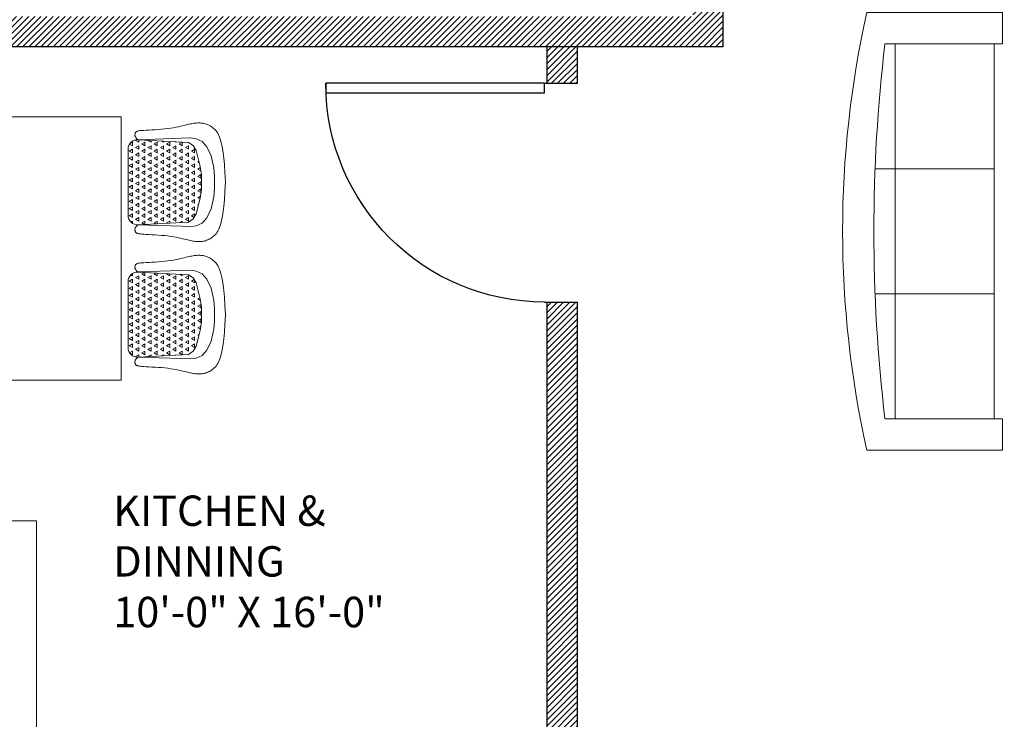
# Model space of a CAD drawing. Units: inches. Extents: x 2443635 to 2446153, y 1826255 to 1827341.
# Tile 8 of 16: x 2444366 to 2444528, y 1826952 to 1827067. Entities that reach past the tile are written whole.
import ezdxf

# ---------------------------------------------------------------- set-up
doc = ezdxf.new("R2010")
doc.units = ezdxf.units.IN
for name, color, linetype, lineweight in [('A-DOOR', 2, 'Continuous', 25), ('A-FLOR-CASE', 8, 'Continuous', 18), ('A-FURN', 6, 'Continuous', 18), ('A-ROOM', 4, 'Continuous', 18), ('A-WALL-INT', 9, 'Continuous', 30), ('A-WALL-PATT', 8, 'Continuous', 13)]:
    doc.layers.add(name, color=color, linetype=linetype, lineweight=lineweight)
doc.styles.get("Standard").update_dxf_attribs({"font": 'arial.ttf'})

# ---------------------------------------------------------------- blocks, each defined once
blk = doc.blocks.new('*X10')
at = {"color": 0}
for p, q in [((152.44, 136.07), (152.22, 136.07)), ((152.35, 136.23), (152.44, 136.07)), ((152.62, 135.75), (152.44, 135.42)), ((152.62, 135.75), (152.81, 135.42)), ((153, 136.4), (152.81, 136.07)), ((153.19, 136.07), (152.81, 136.07)), ((153, 136.4), (153.19, 136.07)), ((153.37, 135.75), (153.19, 135.42)), ((153.37, 135.75), (153.56, 135.42)), ((153.75, 136.4), (153.56, 136.07)), ((153.94, 136.07), (153.56, 136.07)), ((153.75, 136.4), (153.94, 136.07)), ((154.12, 135.75), (153.94, 135.42)), ((154.12, 135.75), (154.31, 135.42)), ((154.5, 136.4), (154.31, 136.07)), ((154.69, 136.07), (154.31, 136.07)), ((154.5, 136.4), (154.69, 136.07)), ((154.87, 135.75), (154.69, 135.42)), ((154.87, 135.75), (155.06, 135.42)), ((155.25, 136.4), (155.06, 136.07)), ((155.44, 136.07), (155.06, 136.07)), ((155.25, 136.4), (155.44, 136.07)), ((155.62, 135.75), (155.44, 135.42)), ((155.62, 135.75), (155.81, 135.42)), ((156, 136.4), (155.81, 136.07)), ((156.19, 136.07), (155.81, 136.07)), ((156, 136.4), (156.19, 136.07)), ((156.37, 135.75), (156.19, 135.42)), ((156.37, 135.75), (156.56, 135.42)), ((156.75, 136.4), (156.56, 136.07)), ((156.94, 136.07), (156.56, 136.07)), ((156.75, 136.4), (156.94, 136.07)), ((157.12, 135.75), (156.94, 135.42)), ((157.12, 135.75), (157.31, 135.42)), ((157.5, 136.4), (157.31, 136.07)), ((157.69, 136.07), (157.31, 136.07)), ((157.5, 136.4), (157.69, 136.07)), ((157.87, 135.75), (157.69, 135.42)), ((157.87, 135.75), (158.06, 135.42)), ((158.25, 136.4), (158.06, 136.07)), ((158.44, 136.07), (158.06, 136.07)), ((158.25, 136.4), (158.44, 136.07)), ((158.62, 135.75), (158.44, 135.42)), ((158.62, 135.75), (158.81, 135.42)), ((159, 136.4), (158.81, 136.07)), ((159.19, 136.07), (158.81, 136.07)), ((159, 136.4), (159.19, 136.07)), ((159.37, 135.75), (159.19, 135.42)), ((159.37, 135.75), (159.56, 135.42)), ((159.75, 136.4), (159.56, 136.07)), ((159.94, 136.07), (159.56, 136.07)), ((159.75, 136.4), (159.94, 136.07)), ((160.12, 135.75), (159.94, 135.42)), ((160.12, 135.75), (160.31, 135.42)), ((160.48, 136.37), (160.31, 136.07)), ((160.69, 136.07), (160.31, 136.07)), ((160.54, 136.33), (160.69, 136.07)), ((160.87, 135.75), (160.69, 135.42)), ((160.87, 135.75), (160.94, 135.64)), ((152.06, 135.44), (152.06, 135.42)), ((152.06, 135.42), (152.06, 135.42)), ((152.25, 135.1), (152.09, 134.82)), ((152.44, 134.78), (152.09, 134.78)), ((152.25, 135.1), (152.44, 134.78)), ((152.81, 135.42), (152.44, 135.42)), ((153, 135.1), (152.81, 134.78)), ((153.19, 134.78), (152.81, 134.78)), ((153, 135.1), (153.19, 134.78)), ((153.56, 135.42), (153.19, 135.42)), ((153.75, 135.1), (153.56, 134.78)), ((153.94, 134.78), (153.56, 134.78)), ((153.75, 135.1), (153.94, 134.78)), ((154.31, 135.42), (153.94, 135.42)), ((154.5, 135.1), (154.31, 134.78)), ((154.69, 134.78), (154.31, 134.78)), ((154.5, 135.1), (154.69, 134.78)), ((155.06, 135.42), (154.69, 135.42)), ((155.25, 135.1), (155.06, 134.78)), ((155.44, 134.78), (155.06, 134.78)), ((155.25, 135.1), (155.44, 134.78)), ((155.81, 135.42), (155.44, 135.42)), ((156, 135.1), (155.81, 134.78)), ((156.19, 134.78), (155.81, 134.78)), ((156, 135.1), (156.19, 134.78)), ((156.56, 135.42), (156.19, 135.42)), ((156.75, 135.1), (156.56, 134.78)), ((156.94, 134.78), (156.56, 134.78)), ((156.75, 135.1), (156.94, 134.78)), ((157.31, 135.42), (156.94, 135.42)), ((157.5, 135.1), (157.31, 134.78)), ((157.69, 134.78), (157.31, 134.78)), ((157.5, 135.1), (157.69, 134.78)), ((158.06, 135.42), (157.69, 135.42)), ((158.25, 135.1), (158.06, 134.78)), ((158.44, 134.78), (158.06, 134.78)), ((158.25, 135.1), (158.44, 134.78)), ((158.81, 135.42), (158.44, 135.42)), ((159, 135.1), (158.81, 134.78)), ((159.19, 134.78), (158.81, 134.78)), ((159, 135.1), (159.19, 134.78)), ((159.56, 135.42), (159.19, 135.42)), ((159.75, 135.1), (159.56, 134.78)), ((159.94, 134.78), (159.56, 134.78)), ((159.75, 135.1), (159.94, 134.78)), ((160.31, 135.42), (159.94, 135.42)), ((160.5, 135.1), (160.31, 134.78)), ((160.69, 134.78), (160.31, 134.78)), ((160.5, 135.1), (160.69, 134.78)), ((160.94, 135.42), (160.69, 135.42)), ((152.25, 133.8), (152.15, 133.63)), ((152.25, 133.8), (152.44, 133.48)), ((152.62, 134.45), (152.44, 134.13)), ((152.81, 134.13), (152.44, 134.13)), ((152.62, 134.45), (152.81, 134.13)), ((153, 133.8), (152.81, 133.48)), ((153, 133.8), (153.19, 133.48)), ((153.37, 134.45), (153.19, 134.13)), ((153.56, 134.13), (153.19, 134.13)), ((153.37, 134.45), (153.56, 134.13)), ((153.75, 133.8), (153.56, 133.48)), ((153.75, 133.8), (153.94, 133.48)), ((154.12, 134.45), (153.94, 134.13)), ((154.31, 134.13), (153.94, 134.13)), ((154.12, 134.45), (154.31, 134.13)), ((154.5, 133.8), (154.31, 133.48)), ((154.5, 133.8), (154.69, 133.48)), ((154.87, 134.45), (154.69, 134.13)), ((155.06, 134.13), (154.69, 134.13)), ((154.87, 134.45), (155.06, 134.13)), ((155.25, 133.8), (155.06, 133.48)), ((155.25, 133.8), (155.44, 133.48)), ((155.62, 134.45), (155.44, 134.13)), ((155.81, 134.13), (155.44, 134.13)), ((155.62, 134.45), (155.81, 134.13)), ((156, 133.8), (155.81, 133.48)), ((156, 133.8), (156.19, 133.48)), ((156.37, 134.45), (156.19, 134.13)), ((156.56, 134.13), (156.19, 134.13)), ((156.37, 134.45), (156.56, 134.13)), ((156.75, 133.8), (156.56, 133.48)), ((156.75, 133.8), (156.94, 133.48)), ((157.12, 134.45), (156.94, 134.13)), ((157.31, 134.13), (156.94, 134.13)), ((157.12, 134.45), (157.31, 134.13)), ((157.5, 133.8), (157.31, 133.48)), ((157.5, 133.8), (157.69, 133.48)), ((157.87, 134.45), (157.69, 134.13)), ((158.06, 134.13), (157.69, 134.13)), ((157.87, 134.45), (158.06, 134.13)), ((158.25, 133.8), (158.06, 133.48)), ((158.25, 133.8), (158.44, 133.48)), ((158.62, 134.45), (158.44, 134.13)), ((158.81, 134.13), (158.44, 134.13)), ((158.62, 134.45), (158.81, 134.13)), ((159, 133.8), (158.81, 133.48)), ((159, 133.8), (159.19, 133.48)), ((159.37, 134.45), (159.19, 134.13)), ((159.56, 134.13), (159.19, 134.13)), ((159.37, 134.45), (159.56, 134.13)), ((159.75, 133.8), (159.56, 133.48)), ((159.75, 133.8), (159.94, 133.48)), ((160.12, 134.45), (159.94, 134.13)), ((160.31, 134.13), (159.94, 134.13)), ((160.12, 134.45), (160.31, 134.13)), ((160.5, 133.8), (160.31, 133.48)), ((160.5, 133.8), (160.69, 133.48)), ((160.87, 134.45), (160.69, 134.13)), ((160.87, 134.13), (160.69, 134.13)), ((160.87, 134.45), (160.89, 134.43)), ((152.44, 133.48), (152.16, 133.48)), ((152.62, 133.15), (152.44, 132.83)), ((152.81, 132.83), (152.44, 132.83)), ((152.62, 133.15), (152.81, 132.83)), ((153.19, 133.48), (152.81, 133.48)), ((153.37, 133.15), (153.19, 132.83)), ((153.56, 132.83), (153.19, 132.83)), ((153.37, 133.15), (153.56, 132.83)), ((153.94, 133.48), (153.56, 133.48)), ((154.12, 133.15), (153.94, 132.83)), ((154.31, 132.83), (153.94, 132.83)), ((154.12, 133.15), (154.31, 132.83)), ((154.69, 133.48), (154.31, 133.48)), ((154.87, 133.15), (154.69, 132.83)), ((155.06, 132.83), (154.69, 132.83)), ((154.87, 133.15), (155.06, 132.83)), ((155.44, 133.48), (155.06, 133.48)), ((155.62, 133.15), (155.44, 132.83)), ((155.81, 132.83), (155.44, 132.83)), ((155.62, 133.15), (155.81, 132.83)), ((156.19, 133.48), (155.81, 133.48)), ((156.37, 133.15), (156.19, 132.83)), ((156.56, 132.83), (156.19, 132.83)), ((156.37, 133.15), (156.56, 132.83)), ((156.94, 133.48), (156.56, 133.48)), ((157.12, 133.15), (156.94, 132.83)), ((157.31, 132.83), (156.94, 132.83)), ((157.12, 133.15), (157.31, 132.83)), ((157.69, 133.48), (157.31, 133.48)), ((157.87, 133.15), (157.69, 132.83)), ((158.06, 132.83), (157.69, 132.83)), ((157.87, 133.15), (158.06, 132.83)), ((158.44, 133.48), (158.06, 133.48)), ((158.62, 133.15), (158.44, 132.83)), ((158.81, 132.83), (158.44, 132.83)), ((158.62, 133.15), (158.81, 132.83)), ((159.19, 133.48), (158.81, 133.48)), ((159.37, 133.15), (159.19, 132.83)), ((159.56, 132.83), (159.19, 132.83)), ((159.37, 133.15), (159.56, 132.83)), ((159.94, 133.48), (159.56, 133.48)), ((160.12, 133.15), (159.94, 132.83)), ((160.31, 132.83), (159.94, 132.83)), ((160.12, 133.15), (160.31, 132.83)), ((160.69, 133.48), (160.31, 133.48)), ((160.81, 133.05), (160.69, 132.83)), ((160.8, 132.83), (160.69, 132.83)), ((152.25, 132.5), (152.22, 132.44)), ((152.44, 132.18), (152.23, 132.18)), ((152.25, 132.5), (152.44, 132.18)), ((152.62, 131.85), (152.44, 131.53)), ((152.81, 131.53), (152.44, 131.53)), ((152.62, 131.85), (152.81, 131.53)), ((153, 132.5), (152.81, 132.18)), ((153.19, 132.18), (152.81, 132.18)), ((153, 132.5), (153.19, 132.18)), ((153.37, 131.85), (153.19, 131.53)), ((153.56, 131.53), (153.19, 131.53)), ((153.37, 131.85), (153.56, 131.53)), ((153.75, 132.5), (153.56, 132.18)), ((153.94, 132.18), (153.56, 132.18)), ((153.75, 132.5), (153.94, 132.18)), ((154.12, 131.85), (153.94, 131.53)), ((154.31, 131.53), (153.94, 131.53)), ((154.12, 131.85), (154.31, 131.53)), ((154.5, 132.5), (154.31, 132.18)), ((154.69, 132.18), (154.31, 132.18)), ((154.5, 132.5), (154.69, 132.18)), ((154.87, 131.85), (154.69, 131.53)), ((155.06, 131.53), (154.69, 131.53)), ((154.87, 131.85), (155.06, 131.53)), ((155.25, 132.5), (155.06, 132.18)), ((155.44, 132.18), (155.06, 132.18)), ((155.25, 132.5), (155.44, 132.18)), ((155.62, 131.85), (155.44, 131.53)), ((155.81, 131.53), (155.44, 131.53)), ((155.62, 131.85), (155.81, 131.53)), ((156, 132.5), (155.81, 132.18)), ((156.19, 132.18), (155.81, 132.18)), ((156, 132.5), (156.19, 132.18)), ((156.37, 131.85), (156.19, 131.53)), ((156.56, 131.53), (156.19, 131.53)), ((156.37, 131.85), (156.56, 131.53)), ((156.75, 132.5), (156.56, 132.18)), ((156.94, 132.18), (156.56, 132.18)), ((156.75, 132.5), (156.94, 132.18)), ((157.12, 131.85), (156.94, 131.53)), ((157.31, 131.53), (156.94, 131.53)), ((157.12, 131.85), (157.31, 131.53)), ((157.5, 132.5), (157.31, 132.18)), ((157.69, 132.18), (157.31, 132.18)), ((157.5, 132.5), (157.69, 132.18)), ((157.87, 131.85), (157.69, 131.53)), ((158.06, 131.53), (157.69, 131.53)), ((157.87, 131.85), (158.06, 131.53)), ((158.25, 132.5), (158.06, 132.18)), ((158.44, 132.18), (158.06, 132.18)), ((158.25, 132.5), (158.44, 132.18)), ((158.62, 131.85), (158.44, 131.53)), ((158.81, 131.53), (158.44, 131.53)), ((158.62, 131.85), (158.81, 131.53)), ((159, 132.5), (158.81, 132.18)), ((159.19, 132.18), (158.81, 132.18)), ((159, 132.5), (159.19, 132.18)), ((159.37, 131.85), (159.19, 131.53)), ((159.56, 131.53), (159.19, 131.53)), ((159.37, 131.85), (159.56, 131.53)), ((159.75, 132.5), (159.56, 132.18)), ((159.94, 132.18), (159.56, 132.18)), ((159.75, 132.5), (159.94, 132.18)), ((160.12, 131.85), (159.94, 131.53)), ((160.31, 131.53), (159.94, 131.53)), ((160.12, 131.85), (160.31, 131.53)), ((160.5, 132.5), (160.31, 132.18)), ((160.69, 132.18), (160.31, 132.18)), ((160.5, 132.5), (160.69, 132.18)), ((160.74, 131.61), (160.69, 131.53)), ((160.73, 131.53), (160.69, 131.53)), ((152.29, 131.14), (152.44, 130.88)), ((152.44, 130.88), (152.3, 130.88)), ((152.62, 130.55), (152.44, 130.23)), ((152.62, 130.55), (152.81, 130.23)), ((153, 131.2), (152.81, 130.88)), ((153.19, 130.88), (152.81, 130.88)), ((153, 131.2), (153.19, 130.88)), ((153.37, 130.55), (153.19, 130.23)), ((153.37, 130.55), (153.56, 130.23)), ((153.75, 131.2), (153.56, 130.88)), ((153.94, 130.88), (153.56, 130.88)), ((153.75, 131.2), (153.94, 130.88)), ((154.12, 130.55), (153.94, 130.23)), ((154.12, 130.55), (154.31, 130.23)), ((154.5, 131.2), (154.31, 130.88)), ((154.69, 130.88), (154.31, 130.88)), ((154.5, 131.2), (154.69, 130.88)), ((154.87, 130.55), (154.69, 130.23)), ((154.87, 130.55), (155.06, 130.23)), ((155.25, 131.2), (155.06, 130.88)), ((155.44, 130.88), (155.06, 130.88)), ((155.25, 131.2), (155.44, 130.88)), ((155.62, 130.55), (155.44, 130.23)), ((155.62, 130.55), (155.81, 130.23)), ((156, 131.2), (155.81, 130.88)), ((156.19, 130.88), (155.81, 130.88)), ((156, 131.2), (156.19, 130.88)), ((156.37, 130.55), (156.19, 130.23)), ((156.37, 130.55), (156.56, 130.23)), ((156.75, 131.2), (156.56, 130.88)), ((156.94, 130.88), (156.56, 130.88)), ((156.75, 131.2), (156.94, 130.88)), ((157.12, 130.55), (156.94, 130.23)), ((157.12, 130.55), (157.31, 130.23)), ((157.5, 131.2), (157.31, 130.88)), ((157.69, 130.88), (157.31, 130.88)), ((157.5, 131.2), (157.69, 130.88)), ((157.87, 130.55), (157.69, 130.23)), ((157.87, 130.55), (158.06, 130.23)), ((158.25, 131.2), (158.06, 130.88)), ((158.44, 130.88), (158.06, 130.88)), ((158.25, 131.2), (158.44, 130.88)), ((158.62, 130.55), (158.44, 130.23)), ((158.62, 130.55), (158.81, 130.23)), ((159, 131.2), (158.81, 130.88)), ((159.19, 130.88), (158.81, 130.88)), ((159, 131.2), (159.19, 130.88)), ((159.37, 130.55), (159.19, 130.23)), ((159.37, 130.55), (159.56, 130.23)), ((159.75, 131.2), (159.56, 130.88)), ((159.94, 130.88), (159.56, 130.88)), ((159.75, 131.2), (159.94, 130.88)), ((160.12, 130.55), (159.94, 130.23)), ((160.12, 130.55), (160.31, 130.23)), ((160.5, 131.2), (160.31, 130.88)), ((160.69, 130.88), (160.31, 130.88)), ((160.5, 131.2), (160.69, 130.88)), ((152.81, 130.23), (152.44, 130.23)), ((153, 129.9), (152.84, 129.63)), ((153.19, 129.58), (152.93, 129.58)), ((153, 129.9), (153.19, 129.58)), ((153.56, 130.23), (153.19, 130.23)), ((153.75, 129.9), (153.56, 129.58)), ((153.94, 129.58), (153.56, 129.58)), ((153.75, 129.9), (153.94, 129.58)), ((154.31, 130.23), (153.94, 130.23)), ((154.5, 129.9), (154.31, 129.58)), ((154.69, 129.58), (154.31, 129.58)), ((154.5, 129.9), (154.69, 129.58)), ((155.06, 130.23), (154.69, 130.23)), ((155.25, 129.9), (155.06, 129.58)), ((155.44, 129.58), (155.06, 129.58)), ((155.25, 129.9), (155.44, 129.58)), ((155.81, 130.23), (155.44, 130.23)), ((156, 129.9), (155.81, 129.58)), ((156.19, 129.58), (155.81, 129.58)), ((156, 129.9), (156.19, 129.58)), ((156.56, 130.23), (156.19, 130.23)), ((156.75, 129.9), (156.56, 129.58)), ((156.94, 129.58), (156.56, 129.58)), ((156.75, 129.9), (156.94, 129.58)), ((157.31, 130.23), (156.94, 130.23)), ((157.5, 129.9), (157.31, 129.58)), ((157.69, 129.58), (157.31, 129.58)), ((157.5, 129.9), (157.69, 129.58)), ((158.06, 130.23), (157.69, 130.23)), ((158.25, 129.9), (158.06, 129.58)), ((158.44, 129.58), (158.06, 129.58)), ((158.25, 129.9), (158.44, 129.58)), ((158.81, 130.23), (158.44, 130.23)), ((159, 129.9), (158.81, 129.58)), ((159.19, 129.58), (158.81, 129.58)), ((159, 129.9), (159.19, 129.58)), ((159.56, 130.23), (159.19, 130.23)), ((159.75, 129.9), (159.56, 129.58)), ((159.94, 129.58), (159.56, 129.58)), ((159.75, 129.9), (159.94, 129.58)), ((160.31, 130.23), (159.94, 130.23)), ((154.12, 129.25), (154.09, 129.19)), ((154.12, 129.25), (154.17, 129.17)), ((154.87, 129.25), (154.74, 129.02)), ((154.87, 129.25), (155.04, 128.97)), ((155.62, 129.25), (155.44, 128.93)), ((155.81, 128.93), (155.44, 128.93)), ((155.62, 129.25), (155.81, 128.93)), ((156.37, 129.25), (156.19, 128.93)), ((156.56, 128.93), (156.19, 128.93)), ((156.37, 129.25), (156.56, 128.93)), ((157.12, 129.25), (156.94, 128.93)), ((157.31, 128.93), (156.94, 128.93)), ((157.12, 129.25), (157.31, 128.93)), ((157.87, 129.25), (157.69, 128.93)), ((157.87, 129.25), (158.03, 128.98)), ((158.62, 129.25), (158.53, 129.09)), ((158.62, 129.25), (158.69, 129.14))]:
    blk.add_line(p, q, dxfattribs=at)
blk = doc.blocks.new('A$C36D1434F')
at = {"layer": 'A-FURN'}
for p, q in [((0, 534.2), (0, 1334.2)), ((0, 1334.2), (1350, 1334.2)), ((1350, 1334.2), (1350, 534.2)), ((1350, 534.2), (0, 534.2))]:
    blk.add_line(p, q, dxfattribs=at)
for points in [[(117.6, 1418.8), (113.4, 1414.5), (109.3, 1411.1), (105.6, 1408.5), (102.1, 1406.7), (98.8, 1405.6), (95.7, 1404.9), (92.9, 1404.7), (90.4, 1404.8), (88.1, 1405.1), (85.9, 1405.5), (84, 1406.2), (82.3, 1407), (80.7, 1408), (79.3, 1409.1), (78, 1410.4), (76.9, 1411.8), (75.8, 1413.4), (74.8, 1415.4), (73.8, 1418.1), (73, 1421.7), (72.1, 1426.5), (71.4, 1432.7), (70.6, 1440.7), (69.8, 1450.6), (69.1, 1462.6), (68.3, 1476.5), (67.4, 1491.7), (66.5, 1507.9), (65.3, 1524.7), (64.1, 1541.5), (62.6, 1558.1), (60.8, 1574), (58.8, 1588.9), (56.6, 1602.7), (54.2, 1615.4), (51.7, 1627.3), (49.2, 1638.3), (46.8, 1648.5), (44.5, 1657.9), (42.3, 1666.7), (40.3, 1674.8), (38.6, 1682.4), (37.1, 1689.6), (35.8, 1696.3), (34.7, 1702.7), (33.8, 1708.8), (33.1, 1714.7), (32.5, 1720.5), (32.1, 1726.2), (31.9, 1731.8), (32, 1737.5), (32.3, 1743.1), (32.8, 1748.7), (33.7, 1754.3), (34.9, 1760), (36.5, 1765.8), (38.5, 1771.7), (40.9, 1777.6), (43.6, 1783.5), (46.7, 1789.3), (50.2, 1795.1), (54, 1800.6), (58.1, 1806), (62.6, 1811.1), (67.4, 1816), (72.6, 1820.5), (78.3, 1824.8), (84.8, 1828.9), (92, 1832.8), (100.2, 1836.5), (109.5, 1840.1), (119.9, 1843.5), (131.9, 1846.9), (146.1, 1850.2), (163.5, 1853.5), (185.3, 1856.6), (212.3, 1859.7), (245.5, 1862.7), (285.9, 1865.6), (334.5, 1868.4)], [(554.3, 1418.8), (558.6, 1414.5), (562.6, 1411.1), (566.3, 1408.5), (569.9, 1406.7), (573.1, 1405.6), (576.2, 1404.9), (579, 1404.7), (581.5, 1404.8), (583.9, 1405.1), (586, 1405.5), (587.9, 1406.2), (589.6, 1407), (591.2, 1408), (592.6, 1409.1), (593.9, 1410.4), (595.1, 1411.8), (596.2, 1413.4), (597.2, 1415.4), (598.1, 1418.1), (599, 1421.7), (599.8, 1426.5), (600.6, 1432.7), (601.3, 1440.7), (602.1, 1450.6), (602.8, 1462.6), (603.6, 1476.5), (604.5, 1491.7), (605.5, 1507.9), (606.6, 1524.7), (607.9, 1541.5), (609.4, 1558.1), (611.1, 1574), (613.1, 1588.9), (615.3, 1602.7), (617.7, 1615.4), (620.2, 1627.3), (622.7, 1638.3), (625.1, 1648.5), (627.5, 1657.9), (629.6, 1666.7), (631.6, 1674.8), (633.3, 1682.4), (634.8, 1689.6), (636.1, 1696.3), (637.2, 1702.7), (638.1, 1708.8), (638.9, 1714.7), (639.4, 1720.5), (639.8, 1726.2), (640, 1731.8), (640, 1737.5), (639.7, 1743.1), (639.1, 1748.7), (638.2, 1754.3), (637, 1760), (635.4, 1765.8), (633.4, 1771.7), (631.1, 1777.6), (628.3, 1783.5), (625.2, 1789.3), (621.7, 1795.1), (617.9, 1800.6), (613.8, 1806), (609.4, 1811.1), (604.6, 1816), (599.4, 1820.5), (593.6, 1824.8), (587.1, 1828.9), (579.9, 1832.8), (571.7, 1836.5), (562.4, 1840.1), (552, 1843.5), (540.1, 1846.9), (525.8, 1850.2), (508.2, 1853.5), (486.3, 1856.6), (458.9, 1859.7), (425.2, 1862.7), (384.1, 1865.6), (334.5, 1868.4)], [(795.7, 1418.8), (791.4, 1414.5), (787.4, 1411.1), (783.7, 1408.5), (780.1, 1406.7), (776.9, 1405.6), (773.8, 1404.9), (771, 1404.7), (768.5, 1404.8), (766.1, 1405.1), (764, 1405.5), (762.1, 1406.2), (760.4, 1407), (758.8, 1408), (757.4, 1409.1), (756.1, 1410.4), (754.9, 1411.8), (753.8, 1413.4), (752.8, 1415.4), (751.9, 1418.1), (751, 1421.7), (750.2, 1426.5), (749.4, 1432.7), (748.7, 1440.7), (747.9, 1450.6), (747.2, 1462.6), (746.4, 1476.5), (745.5, 1491.7), (744.5, 1507.9), (743.4, 1524.7), (742.1, 1541.5), (740.6, 1558.1), (738.9, 1574), (736.9, 1588.9), (734.7, 1602.7), (732.3, 1615.4), (729.8, 1627.3), (727.3, 1638.3), (724.9, 1648.5), (722.5, 1657.9), (720.4, 1666.7), (718.4, 1674.8), (716.7, 1682.4), (715.2, 1689.6), (713.9, 1696.3), (712.8, 1702.7), (711.9, 1708.8), (711.1, 1714.7), (710.6, 1720.5), (710.2, 1726.2), (710, 1731.8), (710, 1737.5), (710.3, 1743.1), (710.9, 1748.7), (711.8, 1754.3), (713, 1760), (714.6, 1765.8), (716.6, 1771.7), (718.9, 1777.6), (721.7, 1783.5), (724.8, 1789.3), (728.3, 1795.1), (732.1, 1800.6), (736.2, 1806), (740.6, 1811.1), (745.4, 1816), (750.6, 1820.5), (756.4, 1824.8), (762.9, 1828.9), (770.1, 1832.8), (778.3, 1836.5), (787.6, 1840.1), (798, 1843.5), (809.9, 1846.9), (824.2, 1850.2), (841.8, 1853.5), (863.7, 1856.6), (891.1, 1859.7), (924.8, 1862.7), (965.9, 1865.6), (1015.5, 1868.4)], [(1232.4, 1418.8), (1236.6, 1414.5), (1240.7, 1411.1), (1244.4, 1408.5), (1247.9, 1406.7), (1251.2, 1405.6), (1254.3, 1404.9), (1257.1, 1404.7), (1259.6, 1404.8), (1261.9, 1405.1), (1264.1, 1405.5), (1266, 1406.2), (1267.7, 1407), (1269.3, 1408), (1270.7, 1409.1), (1272, 1410.4), (1273.1, 1411.8), (1274.2, 1413.4), (1275.2, 1415.4), (1276.2, 1418.1), (1277, 1421.7), (1277.9, 1426.5), (1278.6, 1432.7), (1279.4, 1440.7), (1280.2, 1450.6), (1280.9, 1462.6), (1281.7, 1476.5), (1282.6, 1491.7), (1283.5, 1507.9), (1284.7, 1524.7), (1285.9, 1541.5), (1287.4, 1558.1), (1289.2, 1574), (1291.2, 1588.9), (1293.4, 1602.7), (1295.8, 1615.4), (1298.3, 1627.3), (1300.8, 1638.3), (1303.2, 1648.5), (1305.5, 1657.9), (1307.7, 1666.7), (1309.7, 1674.8), (1311.4, 1682.4), (1312.9, 1689.6), (1314.2, 1696.3), (1315.3, 1702.7), (1316.2, 1708.8), (1316.9, 1714.7), (1317.5, 1720.5), (1317.9, 1726.2), (1318.1, 1731.8), (1318, 1737.5), (1317.7, 1743.1), (1317.2, 1748.7), (1316.3, 1754.3), (1315.1, 1760), (1313.5, 1765.8), (1311.5, 1771.7), (1309.1, 1777.6), (1306.4, 1783.5), (1303.3, 1789.3), (1299.8, 1795.1), (1296, 1800.6), (1291.9, 1806), (1287.4, 1811.1), (1282.6, 1816), (1277.4, 1820.5), (1271.7, 1824.8), (1265.2, 1828.9), (1258, 1832.8), (1249.8, 1836.5), (1240.5, 1840.1), (1230.1, 1843.5), (1218.1, 1846.9), (1203.9, 1850.2), (1186.5, 1853.5), (1164.7, 1856.6), (1137.7, 1859.7), (1104.5, 1862.7), (1064.1, 1865.6), (1015.5, 1868.4)], [(117.6, 1418.8), (110.4, 1641.6), (108.9, 1691.2), (113.4, 1718.2), (127, 1748.3), (154, 1773.8), (200.6, 1794.9), (262.2, 1808.4), (304.3, 1812.9), (337.4, 1812.9)], [(554.3, 1418.8), (561.5, 1641.6), (563, 1691.2), (558.5, 1718.2), (545, 1748.3), (517.9, 1773.8), (471.3, 1794.9), (409.7, 1808.4), (367.6, 1812.9), (334.5, 1812.9)], [(795.7, 1418.8), (788.5, 1641.6), (787, 1691.2), (791.5, 1718.2), (805, 1748.3), (832.1, 1773.8), (878.7, 1794.9), (940.3, 1808.4), (982.4, 1812.9), (1015.5, 1812.9)], [(1232.4, 1418.8), (1239.6, 1641.6), (1241.1, 1691.2), (1236.6, 1718.2), (1223, 1748.3), (1196, 1773.8), (1149.4, 1794.9), (1087.8, 1808.4), (1045.7, 1812.9), (1012.6, 1812.9)], [(117.6, 449.6), (113.4, 453.9), (109.3, 457.3), (105.6, 459.9), (102.1, 461.7), (98.8, 462.8), (95.7, 463.5), (92.9, 463.7), (90.4, 463.6), (88.1, 463.3), (85.9, 462.9), (84, 462.2), (82.3, 461.4), (80.7, 460.4), (79.3, 459.3), (78, 458), (76.9, 456.6), (75.8, 455), (74.8, 453), (73.8, 450.3), (73, 446.7), (72.1, 441.9), (71.4, 435.6), (70.6, 427.7), (69.8, 417.8), (69.1, 405.8), (68.3, 391.9), (67.4, 376.7), (66.5, 360.5), (65.3, 343.7), (64.1, 326.9), (62.6, 310.3), (60.8, 294.4), (58.8, 279.5), (56.6, 265.7), (54.2, 252.9), (51.7, 241.1), (49.2, 230.1), (46.8, 219.9), (44.5, 210.5), (42.3, 201.7), (40.3, 193.6), (38.6, 186), (37.1, 178.8), (35.8, 172.1), (34.7, 165.7), (33.8, 159.6), (33.1, 153.7), (32.5, 147.9), (32.1, 142.2), (31.9, 136.6), (32, 130.9), (32.3, 125.3), (32.8, 119.7), (33.7, 114.1), (34.9, 108.4), (36.5, 102.6), (38.5, 96.7), (40.9, 90.8), (43.6, 84.9), (46.7, 79.1), (50.2, 73.3), (54, 67.8), (58.1, 62.4), (62.6, 57.3), (67.4, 52.4), (72.6, 47.9), (78.3, 43.6), (84.8, 39.5), (92, 35.6), (100.2, 31.9), (109.5, 28.3), (119.9, 24.8), (131.9, 21.5), (146.1, 18.2), (163.5, 14.9), (185.3, 11.8), (212.3, 8.7), (245.5, 5.7), (285.9, 2.8), (334.5, 0)], [(554.3, 449.6), (558.6, 453.9), (562.6, 457.3), (566.3, 459.9), (569.9, 461.7), (573.1, 462.8), (576.2, 463.5), (579, 463.7), (581.5, 463.6), (583.9, 463.3), (586, 462.9), (587.9, 462.2), (589.6, 461.4), (591.2, 460.4), (592.6, 459.3), (593.9, 458), (595.1, 456.6), (596.2, 455), (597.2, 453), (598.1, 450.3), (599, 446.7), (599.8, 441.9), (600.6, 435.6), (601.3, 427.7), (602.1, 417.8), (602.8, 405.8), (603.6, 391.9), (604.5, 376.7), (605.5, 360.5), (606.6, 343.7), (607.9, 326.9), (609.4, 310.3), (611.1, 294.4), (613.1, 279.5), (615.3, 265.7), (617.7, 252.9), (620.2, 241.1), (622.7, 230.1), (625.1, 219.9), (627.5, 210.5), (629.6, 201.7), (631.6, 193.6), (633.3, 186), (634.8, 178.8), (636.1, 172.1), (637.2, 165.7), (638.1, 159.6), (638.9, 153.7), (639.4, 147.9), (639.8, 142.2), (640, 136.6), (640, 130.9), (639.7, 125.3), (639.1, 119.7), (638.2, 114.1), (637, 108.4), (635.4, 102.6), (633.4, 96.7), (631.1, 90.8), (628.3, 84.9), (625.2, 79.1), (621.7, 73.3), (617.9, 67.8), (613.8, 62.4), (609.4, 57.3), (604.6, 52.4), (599.4, 47.9), (593.6, 43.6), (587.1, 39.5), (579.9, 35.6), (571.7, 31.9), (562.4, 28.3), (552, 24.8), (540.1, 21.5), (525.8, 18.2), (508.2, 14.9), (486.3, 11.8), (458.9, 8.7), (425.2, 5.7), (384.1, 2.8), (334.5, 0)], [(795.7, 449.6), (791.4, 453.9), (787.4, 457.3), (783.7, 459.9), (780.1, 461.7), (776.9, 462.8), (773.8, 463.5), (771, 463.7), (768.5, 463.6), (766.1, 463.3), (764, 462.9), (762.1, 462.2), (760.4, 461.4), (758.8, 460.4), (757.4, 459.3), (756.1, 458), (754.9, 456.6), (753.8, 455), (752.8, 453), (751.9, 450.3), (751, 446.7), (750.2, 441.9), (749.4, 435.6), (748.7, 427.7), (747.9, 417.8), (747.2, 405.8), (746.4, 391.9), (745.5, 376.7), (744.5, 360.5), (743.4, 343.7), (742.1, 326.9), (740.6, 310.3), (738.9, 294.4), (736.9, 279.5), (734.7, 265.7), (732.3, 252.9), (729.8, 241.1), (727.3, 230.1), (724.9, 219.9), (722.5, 210.5), (720.4, 201.7), (718.4, 193.6), (716.7, 186), (715.2, 178.8), (713.9, 172.1), (712.8, 165.7), (711.9, 159.6), (711.1, 153.7), (710.6, 147.9), (710.2, 142.2), (710, 136.6), (710, 130.9), (710.3, 125.3), (710.9, 119.7), (711.8, 114.1), (713, 108.4), (714.6, 102.6), (716.6, 96.7), (718.9, 90.8), (721.7, 84.9), (724.8, 79.1), (728.3, 73.3), (732.1, 67.8), (736.2, 62.4), (740.6, 57.3), (745.4, 52.4), (750.6, 47.9), (756.4, 43.6), (762.9, 39.5), (770.1, 35.6), (778.3, 31.9), (787.6, 28.3), (798, 24.8), (809.9, 21.5), (824.2, 18.2), (841.8, 14.9), (863.7, 11.8), (891.1, 8.7), (924.8, 5.7), (965.9, 2.8), (1015.5, 0)], [(1232.4, 449.6), (1236.6, 453.9), (1240.7, 457.3), (1244.4, 459.9), (1247.9, 461.7), (1251.2, 462.8), (1254.3, 463.5), (1257.1, 463.7), (1259.6, 463.6), (1261.9, 463.3), (1264.1, 462.9), (1266, 462.2), (1267.7, 461.4), (1269.3, 460.4), (1270.7, 459.3), (1272, 458), (1273.1, 456.6), (1274.2, 455), (1275.2, 453), (1276.2, 450.3), (1277, 446.7), (1277.9, 441.9), (1278.6, 435.6), (1279.4, 427.7), (1280.2, 417.8), (1280.9, 405.8), (1281.7, 391.9), (1282.6, 376.7), (1283.5, 360.5), (1284.7, 343.7), (1285.9, 326.9), (1287.4, 310.3), (1289.2, 294.4), (1291.2, 279.5), (1293.4, 265.7), (1295.8, 252.9), (1298.3, 241.1), (1300.8, 230.1), (1303.2, 219.9), (1305.5, 210.5), (1307.7, 201.7), (1309.7, 193.6), (1311.4, 186), (1312.9, 178.8), (1314.2, 172.1), (1315.3, 165.7), (1316.2, 159.6), (1316.9, 153.7), (1317.5, 147.9), (1317.9, 142.2), (1318.1, 136.6), (1318, 130.9), (1317.7, 125.3), (1317.2, 119.7), (1316.3, 114.1), (1315.1, 108.4), (1313.5, 102.6), (1311.5, 96.7), (1309.1, 90.8), (1306.4, 84.9), (1303.3, 79.1), (1299.8, 73.3), (1296, 67.8), (1291.9, 62.4), (1287.4, 57.3), (1282.6, 52.4), (1277.4, 47.9), (1271.7, 43.6), (1265.2, 39.5), (1258, 35.6), (1249.8, 31.9), (1240.5, 28.3), (1230.1, 24.8), (1218.1, 21.5), (1203.9, 18.2), (1186.5, 14.9), (1164.7, 11.8), (1137.7, 8.7), (1104.5, 5.7), (1064.1, 2.8), (1015.5, 0)], [(117.6, 449.6), (110.4, 226.8), (108.9, 177.2), (113.4, 150.2), (127, 120.1), (154, 94.6), (200.6, 73.5), (262.2, 60), (304.3, 55.5), (337.4, 55.5)], [(554.3, 449.6), (561.5, 226.8), (563, 177.2), (558.5, 150.2), (545, 120.1), (517.9, 94.6), (471.3, 73.5), (409.7, 60), (367.6, 55.5), (334.5, 55.5)], [(795.7, 449.6), (788.5, 226.8), (787, 177.2), (791.5, 150.2), (805, 120.1), (832.1, 94.6), (878.7, 73.5), (940.3, 60), (982.4, 55.5), (1015.5, 55.5)], [(1232.4, 449.6), (1239.6, 226.8), (1241.1, 177.2), (1236.6, 150.2), (1223, 120.1), (1196, 94.6), (1149.4, 73.5), (1087.8, 60), (1045.7, 55.5), (1012.6, 55.5)]]:
    blk.add_lwpolyline(points, dxfattribs=at)
for points in [[(337.5, 1745.3), (375.1, 1745.3), (417.2, 1739.3), (498.4, 1718.2), (523.9, 1703.2), (540.5, 1679.2), (554.2, 1421.5, -0.429937), (505.2, 1369.7), (166.8, 1369.7, -0.429937), (117.8, 1421.5), (131.6, 1679.2), (148.1, 1703.2), (173.7, 1718.2), (254.8, 1739.3), (296.9, 1745.3), (334.5, 1745.3)], [(1012.5, 1745.3), (974.9, 1745.3), (932.8, 1739.3), (851.6, 1718.2), (826.1, 1703.2), (809.5, 1679.2), (795.8, 1421.5, 0.429937), (844.8, 1369.7), (1183.2, 1369.7, 0.429937), (1232.2, 1421.5), (1218.4, 1679.2), (1201.9, 1703.2), (1176.3, 1718.2), (1095.2, 1739.3), (1053.1, 1745.3), (1015.5, 1745.3)], [(337.5, 123.1), (375.1, 123.1), (417.2, 129.1), (498.4, 150.2), (523.9, 165.2), (540.5, 189.2), (554.2, 446.9, 0.429937), (505.2, 498.7), (166.8, 498.7, 0.429937), (117.8, 446.9), (131.6, 189.2), (148.1, 165.2), (173.7, 150.2), (254.8, 129.1), (296.9, 123.1), (334.5, 123.1)], [(1012.5, 123.1), (974.9, 123.1), (932.8, 129.1), (851.6, 150.2), (826.1, 165.2), (809.5, 189.2), (795.8, 446.9, -0.429937), (844.8, 498.7), (1183.2, 498.7, -0.429937), (1232.2, 446.9), (1218.4, 189.2), (1201.9, 165.2), (1176.3, 150.2), (1095.2, 129.1), (1053.1, 123.1), (1015.5, 123.1)]]:
    blk.add_lwpolyline(points, format="xyb", dxfattribs=at)
at = {"layer": 'A-FURN', "xscale": 49.09090909079987, "yscale": 49.09090909079987, "zscale": 49.09090909079987, "rotation": 180}
blk.add_blockref('*X10', (8018.7, 8071.8), dxfattribs=at)
at = {"layer": 'A-FURN', "extrusion": (0, 0, -1), "xscale": 49.09090909079987, "yscale": 49.09090909079987, "zscale": -49.09090909079999, "rotation": 180}
blk.add_blockref('*X10', (6668.7, 8071.8), dxfattribs=at)
at = {"layer": 'A-FURN', "extrusion": (0, 0, -1), "xscale": 49.09090909079987, "yscale": 49.09090909079987, "zscale": -49.09090909079999}
blk.add_blockref('*X10', (-8018.7, -6203.4), dxfattribs=at)
at = {"layer": 'A-FURN', "xscale": 49.09090909079987, "yscale": 49.09090909079987, "zscale": 49.09090909079987}
blk.add_blockref('*X10', (-6668.7, -6203.4), dxfattribs=at)
blk = doc.blocks.new('*U2')
for p, q in [((0, 0), (0, -6)), ((40, 0), (40, -6))]:
    blk.add_line(p, q)
blk.add_lwpolyline([(0, 0), (0, 40), (1.75, 40), (1.75, 0)], close=True)
blk.add_arc((0, 0), 40, 0, 90)
blk = doc.blocks.new('SOFA-3-SEAT')
at = {"transparency": 33554687}
for p, q in [((0, 22.29), (0, 0)), ((72, 0), (72, 22.29)), ((25.71, 1.34), (25.71, 20.94)), ((46.29, 1.34), (46.29, 20.94)), ((5.14, 0), (5.14, 19.31)), ((66.86, 0), (66.86, 19.31)), ((66.86, 17.67), (5.14, 17.67)), ((0, 0), (5.14, 0)), ((66.86, 1.34), (5.14, 1.34)), ((66.86, 0), (72, 0))]:
    blk.add_line(p, q, dxfattribs=at)
for centre, radius, start, end in [((36, -137.71), 164, 77.3196, 102.6804), ((36, -239.71), 260.86, 83.2065, 96.7935)]:
    blk.add_arc(centre, radius, start, end, dxfattribs=at)
blk = doc.blocks.new('BASE-CABINET-L-PLAN')
at = {"transparency": 33554687}
for p, q in [((0, 78), (36, 78)), ((36, 0), (36, 78)), ((120, 0), (36, 0))]:
    blk.add_line(p, q, dxfattribs=at)

msp = doc.modelspace()

# ---------------------------------------------------------------- hatches: boundary and pattern name
at = {"layer": 'A-WALL-PATT'}
h = msp.add_hatch(dxfattribs=at)
h.set_pattern_fill('JIS_WOOD', color=256)
h.paths.add_polyline_path([(2444481.553, 1827095.288), (2444476.553, 1827095.288), (2444476.553, 1827067.288), (2444332.553, 1827067.288), (2444332.553, 1827062.288), (2444481.553, 1827062.288)])
h.paths.add_polyline_path([(2444457.553, 1827020.288), (2444452.553, 1827020.288), (2444452.553, 1826870.288), (2444457.553, 1826870.288), (2444457.553, 1826930.288), (2444530.053, 1826930.288), (2444530.053, 1826935.288), (2444457.553, 1826935.288)])
h.paths.add_polyline_path([(2444457.553, 1827062.288), (2444452.553, 1827062.288), (2444452.553, 1827056.288), (2444457.553, 1827056.288)])
h.paths.add_polyline_path([(2444638.553, 1826935.288), (2444566.053, 1826935.288), (2444566.053, 1826930.288), (2444638.553, 1826930.288)])
h.paths.add_polyline_path([(2444638.553, 1827152.288), (2444518.553, 1827152.288), (2444518.553, 1827156.288), (2444513.553, 1827156.288), (2444513.553, 1827147.288), (2444638.553, 1827147.288)])
h.paths.add_polyline_path([(2444518.553, 1827296.288), (2444513.553, 1827296.288), (2444513.553, 1827224.288), (2444507.553, 1827224.288), (2444507.553, 1827223.788), (2444507.553, 1827219.288), (2444513.553, 1827219.288), (2444513.553, 1827192.288), (2444518.553, 1827192.288)])
h.paths.add_polyline_path([(2444477.553, 1827223.788, -0.0041669), (2444477.557, 1827224.288), (2444457.553, 1827224.288), (2444457.553, 1827296.288), (2444452.553, 1827296.288), (2444452.553, 1827192.288), (2444457.553, 1827192.288), (2444457.553, 1827219.288), (2444477.553, 1827219.288)])
h.paths.add_polyline_path([(2444481.553, 1827152.288), (2444332.553, 1827152.288), (2444332.553, 1827147.288), (2444476.553, 1827147.288), (2444476.553, 1827137.288), (2444481.553, 1827137.288)])

# ---------------------------------------------------------------- linework, layer by layer
at = {"layer": 'A-WALL-INT'}
for p, q in [((2444481.553, 1827062.288), (2444481.553, 1827095.288)), ((2444481.553, 1827062.288), (2444332.553, 1827062.288)), ((2444452.553, 1827056.288), (2444452.553, 1827062.288)), ((2444457.553, 1827056.288), (2444457.553, 1827062.288)), ((2444452.553, 1826870.288), (2444452.553, 1827020.288)), ((2444457.553, 1826935.288), (2444457.553, 1827020.288))]:
    msp.add_line(p, q, dxfattribs=at)

# ---------------------------------------------------------------- block references
at = {"layer": 'A-DOOR', "xscale": -0.9, "yscale": 0.9, "zscale": 0.9, "rotation": 90}
msp.add_blockref('*U2', (2444452.153, 1827056.288), dxfattribs=at)
at = {"layer": 'A-FLOR-CASE', "transparency": 33554687}
msp.add_blockref('BASE-CABINET-L-PLAN', (2444332.553, 1826906.288), dxfattribs=at)
at = {"layer": 'A-FURN', "transparency": 33554687, "rotation": 89.99999999977271}
msp.add_blockref('SOFA-3-SEAT', (2444527.473, 1826995.927), dxfattribs=at)
at = {"layer": 'A-FURN', "xscale": 0.032113081480791, "yscale": 0.032113081480791, "zscale": 0.032113081480791, "rotation": 270}
msp.add_blockref('A$C36D1434F', (2444339.652, 1827050.79), dxfattribs=at)

# ---------------------------------------------------------------- texts
at = {"layer": 'A-ROOM', "insert": (2444381.193, 1826988.457), "char_height": 5, "attachment_point": 1}
msp.add_mtext_dynamic_manual_height_columns('KITCHEN &\\PDINNING\\P10\'-0" X 16\'-0"', width=52.37406, gutter_width=12.5, heights=[0], dxfattribs=at)

doc.saveas('drawing.dxf')
